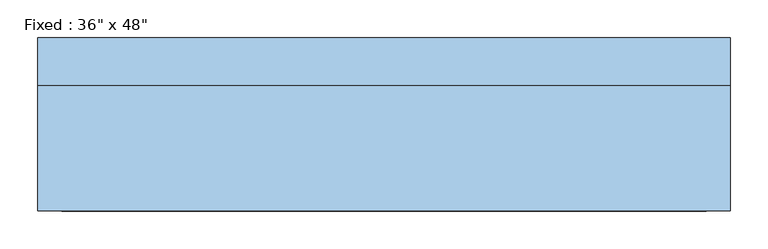
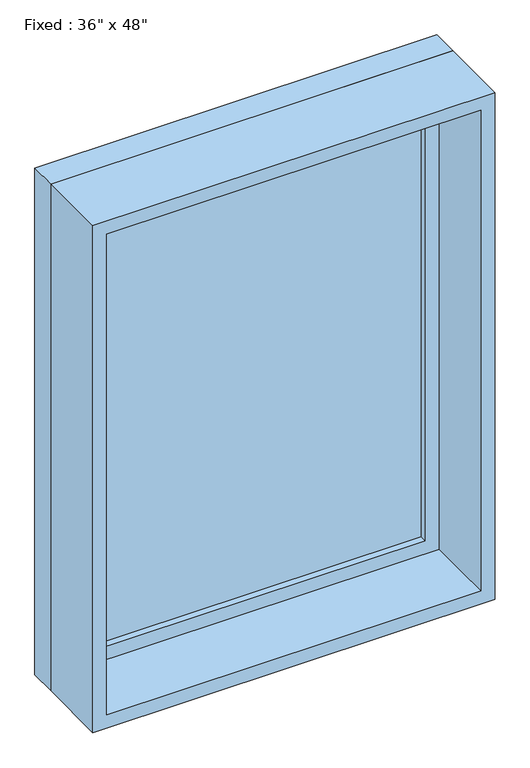
"""IFC4 building model written with IfcOpenShell, lengths in millimetres: window geometry."""

from ifc_helpers import new_model, si_unit, frame, origin, place, context, project, spatial, polyline, outline, extrude, source, transform, mapped, element, save


def window_c1f32544(model_context):
    return source(origin(), model_context, "Body", "SweptSolid", [
        extrude(outline(polyline([(355.6, 66.675), (-431.8, 66.675), (-431.8, 79.375), (355.6, 79.375), (355.6, 66.675)])), frame((0.0, 0.0, 977.9), z_axis=(0.0, 0.0, 1.0), x_axis=(1.0, 0.0, 0.0)), (0.0, 0.0, 1.0), 1092.2),
        extrude(outline(polyline([(2114.55, -476.25), (933.45, -476.25), (933.45, 400.05), (2114.55, 400.05), (2114.55, -476.25)]), holes=[polyline([(2070.1, -431.8), (2070.1, 355.6), (977.9, 355.6), (977.9, -431.8), (2070.1, -431.8)])]), frame((0.0, 50.8, 0.0), z_axis=(0.0, 1.0, 0.0), x_axis=(0.0, 0.0, 1.0)), (0.0, 0.0, 1.0), 44.45),
        extrude(outline(polyline([(2133.6, -495.3), (914.4, -495.3), (914.4, 419.1), (2133.6, 419.1), (2133.6, -495.3)]), holes=[polyline([(2101.85, -463.55), (2101.85, 387.35), (946.15, 387.35), (946.15, -463.55), (2101.85, -463.55)])]), frame((0.0, -114.3, 0.0), z_axis=(0.0, 1.0, 0.0), x_axis=(0.0, 0.0, 1.0)), (0.0, 0.0, 1.0), 165.1),
        extrude(outline(polyline([(2133.6, 419.1), (2133.6, -495.3), (914.4, -495.3), (914.4, 419.1), (2133.6, 419.1)]), holes=[polyline([(2114.55, 400.05), (933.45, 400.05), (933.45, -476.25), (2114.55, -476.25), (2114.55, 400.05)])]), frame((0.0, 50.8, 0.0), z_axis=(0.0, 1.0, 0.0), x_axis=(0.0, 0.0, 1.0)), (0.0, 0.0, 1.0), 63.5),
    ])


if __name__ == "__main__":
    model = new_model("IFC4")
    model_context = context("Model", 3, world=origin())
    ifc_project = project(units=[si_unit("LENGTHUNIT", "METRE", prefix="MILLI")], contexts=[model_context])
    site = spatial("IfcSite", under=ifc_project)
    building = spatial("IfcBuilding", under=site)
    placement = place(None, origin())
    window_shape = window_c1f32544(model_context)
    element("IfcWindow", 1, ObjectType="Fixed : 36\" x 48\"", at=placement, inside=building, context=model_context, shape_type="MappedRepresentation", body=[
        mapped(window_shape, transform((0.0, 0.0, 0.0), x_axis=(1.0, 0.0, 0.0), y_axis=(0.0, 1.0, 0.0), z_axis=(0.0, 0.0, 1.0))),
    ])
    save(model, "model.ifc")

# Revit data of these elements
# Type "Fixed : 36\" x 48\""
#   Type Mark = "W"
#   Construction Type Id = "GSP4R"
#   Assembly Code = "B2020100"
#   Analytic Construction = "1/8 in Pilkington single glazing"
#   Visual Light Transmittance = 0.9
#   Solar Heat Gain Coefficient = 0.78
#   Heat Transfer Coefficient (U) = 0.6496 BTU/(h·ft²·°F)
#   Height = 4' - 0"
#   Default Sill Height = 3' - 0"
#   Width = 3' - 0"
#   Window Inset = 0' - 0 3/4"
#   Define Thermal Properties by = 1
#   Define Thermal Properties by = 1
#   Glass Pane Material = Glass
#   Sash Material = Sash
#   Wall Closure = (empty or 0)
# Element 1 (IfcWindow, "Fixed : 36\" x 48\"")
#   Materials on its faces: "Sash", "Glass"
# Materials
#   "Glass": class "Glass", colour RGB 0 128 192, transparency 0.75, Description = "Soda Lime Glass", Cost = 0
#   "Sash": class "Wood", colour RGB 224 178 126, transparency 0, Cost = 0
